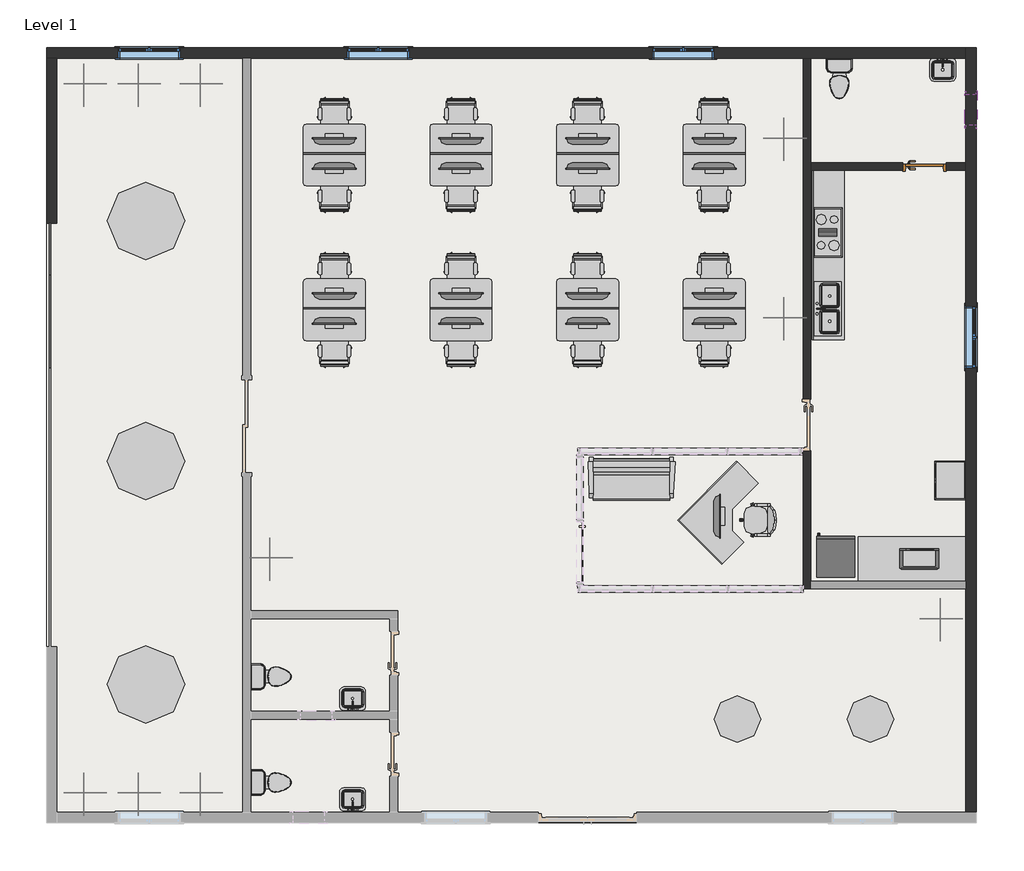
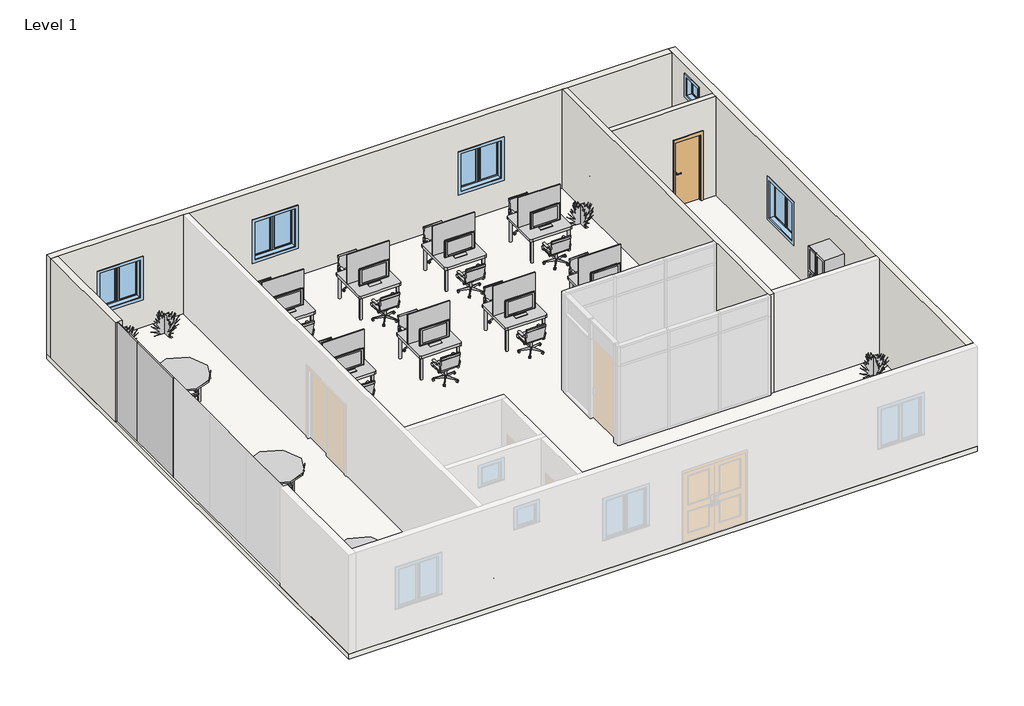
# One storey, part 2 of 2: 52 furniture elements, 10 geographic elements, 10 plates, 7 flow terminals, 5 walls, 5 windows, 3 proxies, 1 door, 1 slab.
# Revit data of these elements (continued)
# Elements 87, 88 (IfcWall, "Generic - 8\"") (continued)
#   Top Offset = 0' - 0"
#   Base Offset = 0' - 0"
#   Unconnected Height = 10' - 0"
#   wall height = 10' - 0"
#   Phase Created = New Construction
#   Base Constraint = Level 1
#   Materials on its faces: "WALL 1", "Metal Door - Red"
# Element 89 (IfcWall, "Generic - 8\"")
#   Top Offset = 0' - 0"
#   Base Offset = 0' - 0"
#   Unconnected Height = 10' - 0"
#   wall height = 10' - 0"
#   Phase Created = New Construction
#   Base Constraint = Level 1
#   Materials on its faces: "Metal Door - Red", "WALL 1"
# Element 90 (IfcWindow, "Casement Dbl with Trim : 48\" x 48\"")
#   Mark = "5"
#   Phase Created = New Construction
#   Materials on its faces: "Sash", "Trim", "Glass"
# Element 91 (IfcWindow, "Casement Dbl with Trim : 48\" x 48\"")
#   Mark = "6"
#   Phase Created = New Construction
#   Materials on its faces: "Sash", "Trim", "Glass"
# Element 92 (IfcWindow, "Casement Dbl with Trim : 48\" x 48\"")
#   Mark = "3"
#   Phase Created = New Construction
#   Materials on its faces: "Sash", "Trim", "Glass"
# Element 93 (IfcWindow, "Casement Dbl with Trim : 48\" x 48\"")
#   Mark = "4"
#   Phase Created = New Construction
#   Materials on its faces: "Sash", "Trim", "Glass"
# Element 94 (IfcWindow, "Transom with Trim : 24\" x 24\"")
#   Mark = "10"
#   Phase Created = New Construction
#   Materials on its faces: "Sash", "Trim", "Glass"
# Materials
#   "Steel, Chrome Plated": class "Metal", colour RGB 17 17 17, transparency 0, Description = "Chromiuim plated steel", Cost = 0
#   "Steel, Polished": class "Metal", colour RGB 57 57 57, transparency 0, Description = "Polished steel", Cost = 0
#   "Laminate, Ivory, Matte": class "Plastic", colour RGB 247 247 239, transparency 0, Description = "Plastic Laminate - Ivory, Matte", Cost = 0
#   "Steel, Paint Finish, Ivory, Glossy": class "Metal", colour RGB 247 247 239, transparency 0, Description = "Steel, paint finish, ivory, glossy", Cost = 0
#   "Wood - Birch": class "Wood", colour RGB 166 116 52, transparency 0, Cost = 0
#   "Metal - Paint Finish - Grey": class "Paint", colour RGB 104 104 104, transparency 0, Cost = 0
#   "Aluminum": class "Metal", colour RGB 247 247 247, transparency 0, Description = "Aluminum 6061", Cost = 0
#   "Porcelain, Linen": class "Ceramic", colour RGB 249 239 230, transparency 0, Description = "Porcelain, linen", Cost = 0
#   "Laminate, Linen, Matte": class "Plastic", colour RGB 249 239 230, transparency 0, Description = "Plastic Laminate - Linen, Matte", Cost = 0
#   "Plastic, Opaque Black": class "Plastic", colour RGB 0 0 0, transparency 0, Description = "Plastic, generic, opaque black", Cost = 0
#   "Textile - Slate Blue": class "Fabric", colour RGB 98 102 118, transparency 0
#   "Cherry": class "Wood", colour RGB 226 177 128, transparency 0, Description = "Prunus Serotina", Cost = 0
#   "Linen, Beige": class "Textile", colour RGB 249 239 230, transparency 0, Description = "Linen, beige", Cost = 0
#   "Pine": class "Wood", colour RGB 223 192 134, transparency 0, Description = "Pinus Echinata", Cost = 0
#   "Birch": class "Wood", colour RGB 224 178 126, transparency 0, Description = "Betula Alleghaniensis", Cost = 0
#   "Cabinets - Handles": class "Metal", colour RGB 57 57 57, transparency 0
#   "WALL 1": class "Generic", colour RGB 120 120 120, transparency 0, Cost = 0
#   "Glass": class "Glass", colour RGB 0 128 192, transparency 0.75, Description = "Soda Lime Glass", Cost = 0
#   "Sash": class "Wood", colour RGB 224 178 126, transparency 0
#   "Trim": class "Wood", colour RGB 224 178 126, transparency 0
#   "Counter Top": class "Wood", colour RGB 226 177 128, transparency 0
#   "TV - Black": colour RGB 49 49 49, transparency 0
#   "TV - Glass": colour RGB 157 157 157, transparency 0.9
#   "TV - Screen": colour RGB 0 0 0, transparency 0
#   "Cabinets": colour RGB 249 249 249, transparency 0
#   "Default Wall": colour RGB 128 128 128, transparency 0
#   "Metal Door - Red": class "Paint", colour RGB 135 0 0, transparency 0, Cost = 0
